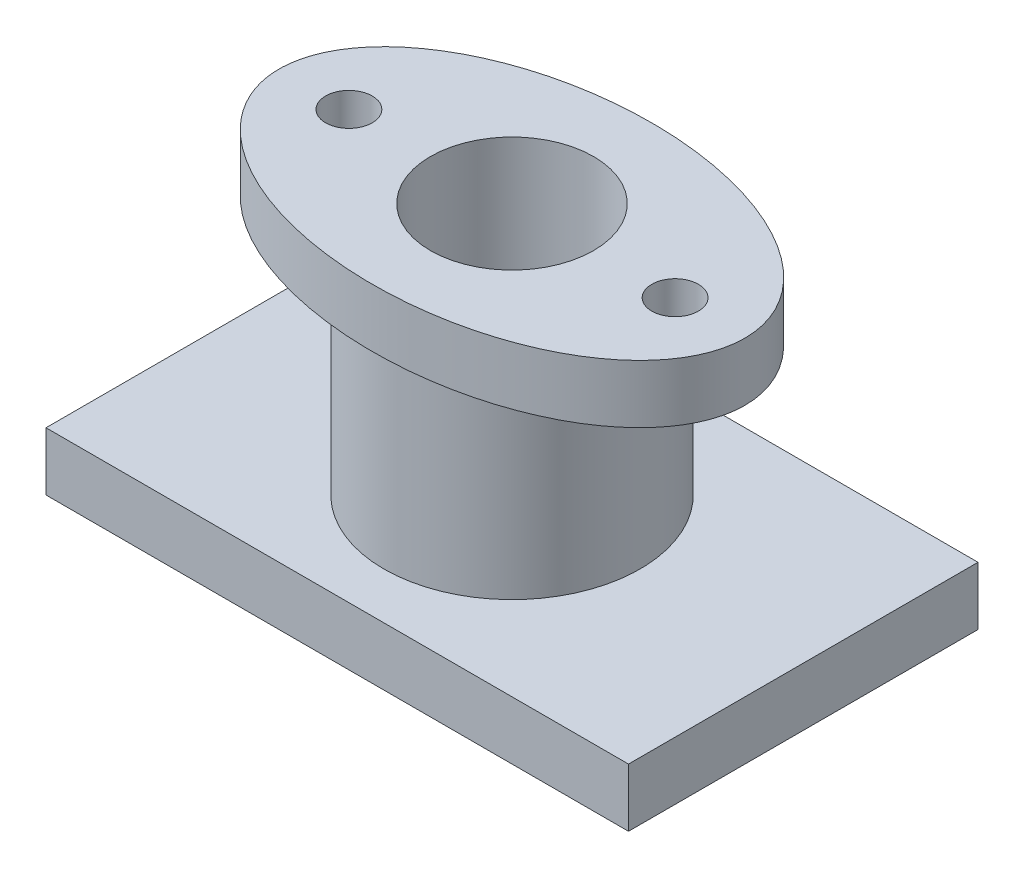
SolidWorks part; units mm, degrees
material "Gray Cast Iron"
ref_plane "Front Plane" through (0, 0, 0) normal (0, 0, 1) x (1, 0, 0)
ref_plane "Top Plane" through (0, 0, 0) normal (0, 1, 0) x (1, 0, 0)
ref_plane "Right Plane" through (0, 0, 0) normal (1, 0, 0) x (0, 0, -1)
sketch "Base Plate Sketch" plane through (0, 0, 0) normal (0, 1, 0) x (1, 0, 0)
  line L1 (-75, -45) -> (75, -45)
  line L2 (-75, -45) -> (-75, 45)
  line L3 (-75, 45) -> (75, 45)
  line L4 (75, -45) -> (75, 45)
  line L5 (-75, -45) -> (75, 45) construction
  line L6 (-75, 45) -> (75, -45) construction
  point P0 (0, 0)
  dimension "D1" = 150
  dimension "D2" = 90
extrude "Base Plate 150x90x15" add sketch "Base Plate Sketch" along normal blind 15
sketch "Boss Tube Sketch" plane through (0, 15, 0) normal (0, 1, 0) x (1, 0, 0)
  circle A0 centre (0, 0) radius 33
  circle A1 centre (0, 0) radius 21
  dimension "D1" = 66
  dimension "D2" = 42
extrude "Boss Tube Ø66" add sketch "Boss Tube Sketch" along normal blind 50
sketch "Oval Flange Sketch" plane through (0, 65, 0) normal (0, 1, 0) x (1, 0, 0)
  line L0 (-95.2391, 0) -> (86.9856, 0) construction
  circle A1 centre (0, 0) radius 21 construction
  circle A2 centre (0, 0) radius 21
  ellipse E0 centre (0, 0) end of major axis (60, 0) minor radius 36
  dimension "D1" = 120
  dimension "D2" = 72
extrude "Oval Flange 120x72" add sketch "Oval Flange Sketch" along normal blind 15
sketch "Base Bore Sketch" plane through (0, 15, 0) normal (0, 1, 0) x (1, 0, 0)
  circle A0 centre (0, 0) radius 16.5
  dimension "D1" = 33
extrude "Base Bore Ø33" cut sketch "Base Bore Sketch" against normal blind 15
sketch "Flange Bolt Hole Sketch" plane through (0, 80, 0) normal (0, 1, 0) x (1, 0, 0)
  line L0 (-60, 0) -> (60, 0) construction
  line L1 (0, 60.1667) -> (0, -57.8101) construction
  circle A0 centre (-41.9958, 0) radius 6
  circle A1 centre (41.9958, 0) radius 6
  ellipse E0 centre (0, 0) end of major axis (60, 0) minor radius 36 construction
  dimension "D1" = 12
  dimension "D2" = 41.9958
extrude "Flange Bolt Hole" cut sketch "Flange Bolt Hole Sketch" against normal blind 15
